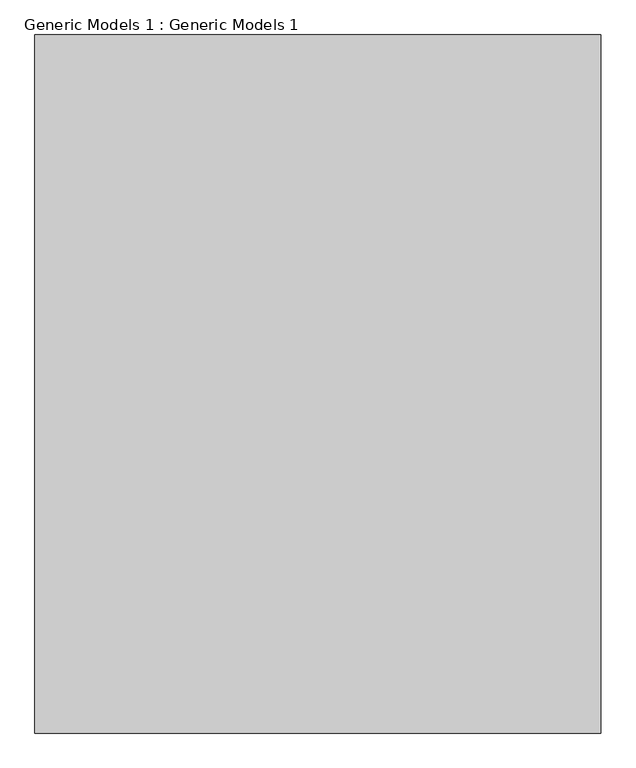
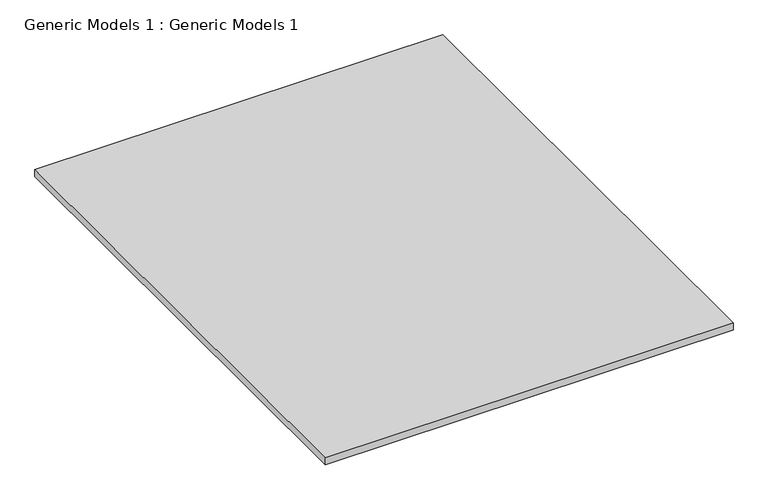
"""IFC4 building model written with IfcOpenShell, lengths in millimetres: proxy geometry, Generic Models 1 : Generic Models 1."""

from ifc_helpers import new_model, si_unit, frame, origin, place, context, project, spatial, polyline, outline, extrude, source, transform, mapped, element, save


def generic_models_1_generic_models_1_f562e270(model_context):
    return source(origin(), model_context, "Body", "SweptSolid", [
        extrude(outline(polyline([(-1831.4052444, -1703.8008704), (-1831.4052444, -23008.0611591), (-19099.2714631, -23008.0611591), (-19099.2714631, -1703.8008704), (-1831.4052444, -1703.8008704)])), frame((0.0, 0.0, -304.8), z_axis=(0.0, 0.0, 1.0), x_axis=(1.0, 0.0, 0.0)), (0.0, 0.0, 1.0), 304.8),
    ])


if __name__ == "__main__":
    model = new_model("IFC4")
    model_context = context("Model", 3, world=origin())
    ifc_project = project(units=[si_unit("LENGTHUNIT", "METRE", prefix="MILLI")], contexts=[model_context])
    site = spatial("IfcSite", under=ifc_project)
    building = spatial("IfcBuilding", under=site)
    placement = place(None, origin())
    generic_models_1_generic_models_1_shape = generic_models_1_generic_models_1_f562e270(model_context)
    element("IfcBuildingElementProxy", 1, Name="Generic Models 1 : Generic Models 1", ObjectType="Generic Models 1 : Generic Models 1", at=placement, inside=building, context=model_context, shape_type="MappedRepresentation", body=[
        mapped(generic_models_1_generic_models_1_shape, transform((0.0, 0.0, 0.0), x_axis=(1.0, 0.0, 0.0), y_axis=(0.0, 1.0, 0.0), z_axis=(0.0, 0.0, 1.0))),
    ])
    save(model, "model.ifc")
